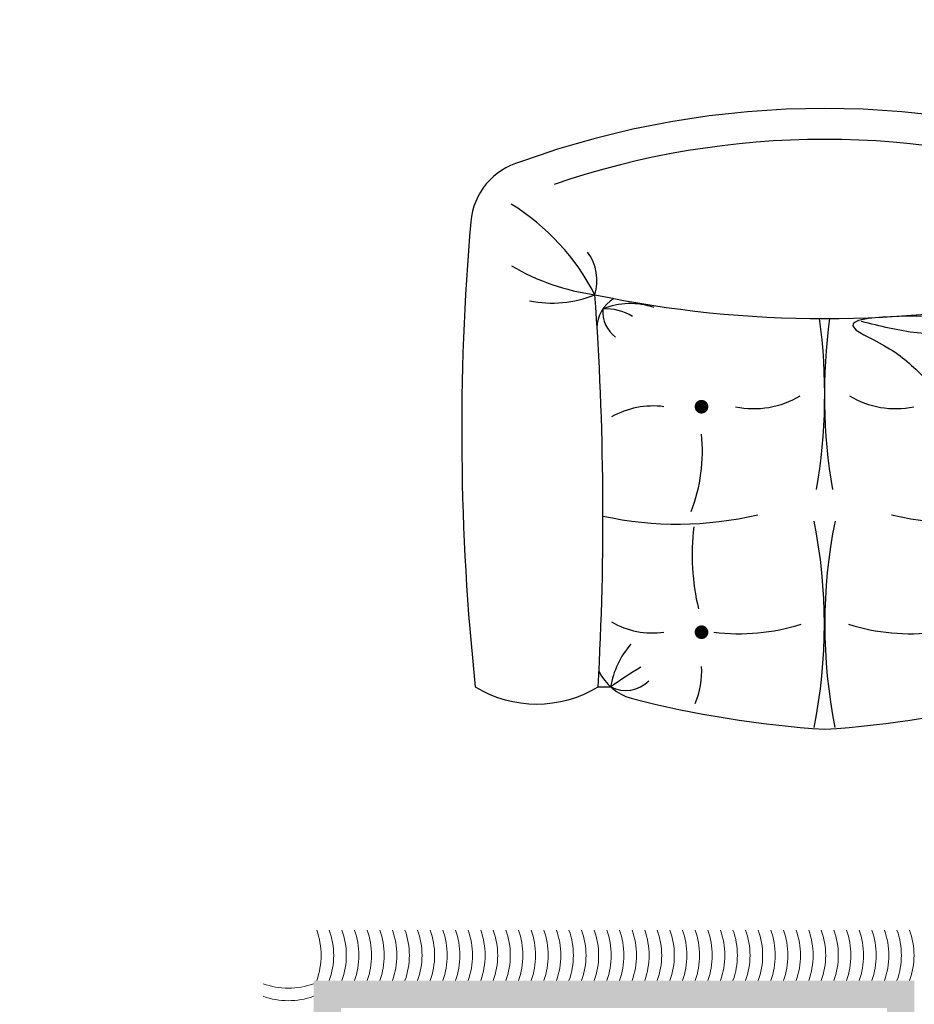
# Model space of a CAD drawing. Units: inches. Extents: x 844 to 2234, y 346 to 1084.
# Tile 88 of 93: x 1990 to 2011, y 713 to 736. Entities that reach past the tile are written whole.
import ezdxf

# ---------------------------------------------------------------- set-up
doc = ezdxf.new("R2010")
doc.units = ezdxf.units.IN
doc.header["$MEASUREMENT"] = 0
for name, color, linetype, lineweight in [('A-ANNO-DIMS', 2, 'Continuous', 18), ('furniture', 8, 'Continuous', 18), ('RA-AP-01$0$INT', 35, 'Continuous', 5)]:
    doc.layers.add(name, color=color, linetype=linetype, lineweight=lineweight)
doc.layers.add('RA-AP-01$0$FURN', color=3, linetype='Continuous')
doc.layers.add('RA-AP-01$0$WOOD', color=64, linetype='Continuous')
doc.styles.get("Standard").update_dxf_attribs({"font": 'arial.ttf'})
doc.dimstyles.get("Standard").update_dxf_attribs({"dimtxt": 6, "dimasz": 3, "dimexe": 0.18, "dimexo": 0.0625, "dimgap": 0.09, "dimtad": 0, "dimtih": 1, "dimtoh": 1, "dimdec": 1, "dimzin": 0, "dimdsep": 46, "dimlunit": 3, "dimtxsty": 'Standard', "dimblk": 'ARCHTICK', "dimcen": 0.09, "dimadec": 0, "dimazin": 0, "dimtfac": 1, "dimtdec": 1, "dimtofl": 0, "dimtmove": 0, "dimatfit": 3, "dimfxl": 1, "dimtolj": 1, "dimtzin": 0, "dimarcsym": 0})

# ---------------------------------------------------------------- blocks, each defined once
blk = doc.blocks.new('A$C18D01794')
at = {"layer": 'RA-AP-01$0$INT'}
h = blk.add_hatch(color=256, dxfattribs=at)
h.paths.add_polyline_path([(4.355206456958071, -6.156712009588037), (4.355206456958071, -8.056712009588038), (5.455206456958072, -8.056712009588038), (5.455206456958072, -6.156712009588037)])
h.paths.add_polyline_path([(4.405206456958072, -8.006712009588039), (4.405206456958072, -6.206712009588038), (5.405206456958072, -6.206712009588038), (5.405206456958072, -8.006712009588039)], flags=16)
for centre, start, end in [((5.501406456971106, -8.156264458284674), 70.20384312943132, 109.796156871843), ((4.492158905671144, -8.102912009578965), 160.2038431286875, 199.7961568711004), ((4.515258905666937, -8.102912009582035), 160.2038431286875, 199.7961568711004), ((4.53835890566273, -8.102912009585104), 160.2038431286875, 199.7961568711004), ((4.561458905665799, -8.102912009585218), 160.2038431286875, 199.7961568711004), ((4.584558905661592, -8.102912009588287), 160.2038431286875, 199.7961568711004), ((4.607658905664661, -8.102912009588401), 160.2038431286875, 199.7961568711004), ((4.630758905664774, -8.102912009585673), 160.2038431286875, 199.7961568711004), ((4.653858905660567, -8.102912009588742), 160.2038431286875, 199.7961568711004), ((4.676958905663636, -8.102912009588856), 160.2038431286875, 199.7961568711004), ((4.700058905663976, -8.102912009589083), 160.2038431286875, 199.7961568711004), ((4.723158905662498, -8.102912009586241), 160.2038431286875, 199.7961568711004), ((4.746258905662839, -8.102912009586355), 160.2038431286875, 199.7961568711004), ((4.769358905662952, -8.102912009589536), 160.2038431286875, 199.7961568711004), ((4.792458905660109, -8.102912009586696), 160.2038431286875, 199.7961568711004), ((4.815558905661814, -8.10291200958681), 160.2038431286875, 199.7961568711004), ((4.838658905662154, -8.102912009587037), 160.2038431286875, 199.7961568711004), ((4.861758905665223, -8.102912009590106), 160.2038431286875, 199.7961568711004), ((4.884858905661016, -8.102912009587264), 160.2038431286875, 199.7961568711004), ((4.907958905662721, -8.102912009587492), 160.2038431286875, 199.7961568711004), ((4.931058905658514, -8.102912009590447), 160.2038431286875, 199.7961568711004), ((4.954158905661583, -8.102912009587717), 160.2038431286875, 199.7961568711004), ((4.977258905663288, -8.102912009587946), 160.2038431286875, 199.7961568711004), ((5.000358905663628, -8.102912009587946), 160.2038431286875, 199.7961568711004), ((5.023458905665333, -8.10291200959113), 160.2038431286875, 199.7961568711004), ((5.046558905660899, -8.102912009588287), 160.2038431286875, 199.7961568711004), ((5.069658905661239, -8.102912009588401), 160.2038431286875, 199.7961568711004), ((5.092758905664308, -8.102912009588628), 160.2038431286875, 199.7961568711004), ((5.115858905663057, -8.102912009585786), 160.2038431286875, 199.7961568711004), ((5.13895890566317, -8.102912009588856), 160.2038431286875, 199.7961568711004), ((5.162058905663511, -8.102912009589083), 160.2038431286875, 199.7961568711004), ((5.185158905659076, -8.102912009589197), 160.2038431286875, 199.7961568711004), ((5.208258905660781, -8.102912009586355), 160.2038431286875, 199.7961568711004), ((5.231358905662486, -8.102912009589536), 160.2038431286875, 199.7961568711004), ((5.254458905661235, -8.102912009589652), 160.2038431286875, 199.7961568711004), ((5.277558905661575, -8.102912009589765), 160.2038431286875, 199.7961568711004), ((5.300658905661689, -8.102912009587037), 160.2038431286875, 199.7961568711004), ((5.323758905658846, -8.10291200958715), 160.2038431286875, 199.7961568711004), ((5.346858905659186, -8.10291200959022), 160.2038431286875, 199.7961568711004), ((5.369958905662255, -8.102912009587492), 160.2038431286875, 199.7961568711004), ((5.39305890566396, -8.102912009587492), 160.2038431286875, 199.7961568711004), ((5.416158905664301, -8.102912009587717), 160.2038431286875, 199.7961568711004), ((5.439258905666005, -8.102912009590902), 160.2038431286875, 199.7961568711004), ((5.462358905661571, -8.102912009587946), 160.2038431286875, 199.7961568711004), ((5.485458905657364, -8.10291200958499), 160.2038431286875, 199.7961568711004), ((5.508558905660433, -8.102912009588287), 160.2038431286875, 199.7961568711004), ((5.531658905655999, -8.102912009585332), 160.2038431286875, 199.7961568711004), ((5.554758905651792, -8.102912009582376), 160.2038431286875, 199.7961568711004), ((5.577858905654861, -8.102912009585673), 160.2038431286875, 199.7961568711004), ((5.501406456971106, -8.179364458283423), 70.20384312943132, 109.796156871843)]:
    blk.add_arc(centre, 0.136414042854523, start, end, dxfattribs=at)
blk = doc.blocks.new('A$C7F4351E2')
at = {"layer": 'RA-AP-01$0$FURN'}
for p, q in [((8.352559572600457, -8.263941955512525), (8.35255957259913, -8.282283310927069)), ((8.352559572600457, -8.927748273106442), (8.35255957259913, -8.909406917691898))]:
    blk.add_line(p, q, dxfattribs=at)
at = {"layer": 'RA-AP-01$0$FURN', "const_width": 0.01}
for points in [[(8.437812509519787, -8.415359762755768, 1), (8.427812509519786, -8.415359762755742, 1)], [(8.758197489244363, -8.415359762756214, -1), (8.768197489244365, -8.415359762756214, -1)], [(8.437812509519787, -8.776330465863198, -1), (8.427812509519786, -8.776330465863225, -1)], [(8.758197489244363, -8.776330465862753, 1), (8.768197489244365, -8.776330465862753, 1)]]:
    blk.add_lwpolyline(points, format="xyb", close=True, dxfattribs=at)
at = {"layer": 'RA-AP-01$0$FURN'}
for centre, radius, start, end in [((8.727559572604601, -11.61690445537682), 3.552808610866049, 85.0473312316413, 96.05887237565803), ((9.025650106946005, -8.176987401637472), 0.1, 15.499494600857, 85.04733123164159), ((8.50205957259015, -8.17394195551301), 0.1744999999876311, 148.9517780040467, 211.048221995953), ((8.77247054904813, -7.958543863781743), 0.3382138395168437, 297.2303327094027, 328.2563708342649), ((9.2484631175852, -8.302692737637487), 0.3241573581843151, 149.2985674842688, 172.3026350986055), ((7.88981694267423, -8.595845114309485), 1.310286319972027, 340.1192502251003, 19.8807497748998), ((9.084915705374858, -8.196040134964925), 0.1698955038956699, 168.877843135945, 201.8512383801196), ((7.929864357850293, -8.595845114309483), 1.224941341589781, 341.1257460634955, 18.87425393650447), ((8.947672844970796, -8.191835192646359), 0.0704710051510922, 253.1338634205325, 306.4126496157095), ((8.408522229993444, -8.33300072568355), 0.0753785023123622, 115.8745619060558, 163.9833547230034), ((8.603635103111959, -3.79706073025477), 4.473931917517753, 266.7828902523826, 274.1477233631118), ((8.878389979098333, -8.312202545234353), 0.05, 30.14777190425723, 89.99999999905349), ((10.52713941284929, -8.595845114309466), 1.634931324962266, 168.1200364254424, 191.8799635745573), ((9.101231010340802, -8.38034106221356), 0.5100538472773755, 167.6182489359307, 193.3122231353938), ((8.903279781571525, -8.31837865610295), 0.0478550828899777, 86.575295631534, 142.6833829238214), ((8.838100984994732, -8.276822957859652), 0.0683206773889159, 326.6729861493449, 5.218395042636973), ((8.810121490949696, -8.31110757721543), 0.1042084262671507, 340.4828318717155, 22.86929393278168), ((8.395364730619693, -8.304213854581548), 0.0479292786975047, 152.8070868543555, 225.4025460716553), ((8.333592787569726, -8.402663469525104), 0.1218651776285568, 48.0375529564433, 81.04623209541253), ((7.439612310514541, -8.913795367824825), 1.11020813118073, 31.93286085977143, 34.66647731879807), ((8.553131949433, -8.344109762755968), 0.1214118203512435, 150.1419074485596, 187.691663289156), ((8.642878049331348, -8.344109762756093), 0.1214118203512435, 352.3083367106845, 29.85809255128089), ((9.82633505008426, -8.696671375220811), 1.539060359583382, 165.5338783218257, 176.2437734318419), ((8.374918524725835, -8.294321202996931), 0.1212957045587361, 247.3375839744822, 273.7314750942433), ((8.546954810732721, -8.753394424755975), 0.3517162425384579, 83.41248966761125, 103.1674570565571), ((8.697701155637269, -8.172468128267624), 0.2442261434243043, 248.9017070735605, 275.9923925191661), ((8.73287643248165, -8.469775898206471), 0.3023568492824586, 173.0944825511667, 197.588060785551), ((8.889871101981017, -8.492307869305423), 0.1295083186917369, 167.9901339202812, 211.3796151021958), ((8.444145567704187, -7.829943385268752), 0.765467899454341, 258.6273206109321, 281.4174148186357), ((9.82633505008426, -8.495018853398156), 1.539060359583382, 183.7562265681581, 194.4661216781742), ((8.444145567704187, -9.361312955433425), 0.765467899454341, 78.58258518136427, 101.3726793890678), ((8.781211457338294, -7.772561243483908), 0.8232838708255751, 260.2449188973366, 277.7495311655964), ((8.781211457338294, -9.418695097218269), 0.8232838708255751, 82.25060502413102, 99.75508110266344), ((8.73287643248165, -8.721914330412496), 0.3023568492824586, 162.411939214449, 186.9055174488332), ((8.889871101981017, -8.699382359313544), 0.1295083186917369, 148.6203848978042, 192.0098660797188), ((9.101231010340802, -8.811349166405407), 0.5100538472773755, 166.6877768646062, 192.3817510640693), ((8.799643412436344, -8.749969313933361), 0.0689028341546707, 265.5384273543114, 353.5804828909086), ((8.374918524725835, -8.897369025622035), 0.1212957045587361, 86.26852490575668, 112.6624160255178), ((8.546954810732721, -8.438295803862992), 0.3517162425384579, 256.8325429434429, 276.5875103323888), ((8.697701155637269, -9.019222100351342), 0.2442261434243043, 84.00760748083387, 111.0982929264395), ((8.553131949433, -8.847580465862999), 0.1214118203512435, 172.308336710844, 209.8580925514404), ((8.395364730619693, -8.88747637403742), 0.0479292786975047, 134.5974539283447, 207.1929131456445), ((8.785133372574222, -8.874256642962408), 0.0310151388417235, 42.62105484496073, 114.2239681486109), ((8.810121490949696, -8.880582651403534), 0.1042084262671507, 337.1307060672183, 19.51716812828453), ((7.439612310514541, -8.277894860794142), 1.11020813118073, 325.333522681202, 328.0671391402286), ((8.408522229993444, -8.858689502935416), 0.0753785023123622, 196.0166452769965, 244.1254380939442), ((8.333592787569726, -8.789026759093863), 0.1218651776285568, 278.9537679045875, 311.9624470435567), ((8.838100984994732, -8.914867270759315), 0.0683206773889159, 354.781604957363, 33.32701385065517), ((8.642878049331348, -8.847580465862874), 0.1214118203512435, 330.1419074487191, 340.3913536181062), ((8.878389979098333, -8.879487683384612), 0.05, 270.0000000009465, 337.4173275753961), ((8.903279781571525, -8.873311572516016), 0.0478550828899777, 217.3166170761785, 273.424704368466), ((8.50205957259015, -9.017748273105955), 0.1744999999876311, 148.9517780040469, 211.0482219959533), ((8.603635103111959, -13.39462949836419), 4.473931917517753, 85.85227663688822, 93.21710974761734), ((9.084915705374858, -8.995650093654042), 0.1698955038956699, 158.1487616198804, 191.122156864055), ((8.947672844970796, -8.999855035972608), 0.0704710051510922, 53.58735038429053, 106.8661365794674), ((8.77247054904813, -9.233146364837223), 0.3382138395168437, 31.74362916573515, 62.76966729059727), ((9.2484631175852, -8.88899749098148), 0.3241573581843151, 187.6973649013944, 210.7014325157311), ((9.025650106946005, -9.014702826981493), 0.1, 274.9526687683584, 344.500505399143), ((8.727559572604601, -5.574785773242145), 3.552808610866049, 263.941127624342, 274.9526687683587)]:
    blk.add_arc(centre, radius, start, end, dxfattribs=at)
for points, knots in [([(8.764421239581775, -8.929562504990262), (8.755250524728652, -8.881106864374377), (8.74196437992213, -8.810906376383404), (8.80604948961138, -8.740469753734786), (8.847474678848357, -8.701097198289744), (8.897142214037096, -8.58322730303861), (8.897091569728207, -8.784804210134517), (8.88612504526093, -8.897825917224484), (8.806539053396843, -8.9185794820093), (8.764421239581775, -8.92956250499026)], [0, 0, 0, 0, 0.1367586589314792, 0.1981301758052368, 0.2677729570689282, 0.3281194902553322, 0.4737578340741565, 0.5765194025309516, 0.6920332287422236, 0.6920332287422236, 0.6920332287422236, 0.6920332287422236]), ([(8.764421239581775, -8.92956250499026), (8.782204778269502, -8.914603263160053), (8.821592007255505, -8.881471326160916), (8.86917941606436, -8.814322636989944), (8.867818990542759, -8.729338202119969), (8.881231406199264, -8.676770566934765), (8.888101821971249, -8.649843164808122)], [0, 0, 0, 0, 0.070018540671015, 0.1550780383534498, 0.2344491945777043, 0.3178048737568289, 0.3178048737568289, 0.3178048737568289, 0.3178048737568289])]:
    blk.add_open_spline(points, degree=3, knots=knots, dxfattribs=at)
blk = doc.blocks.new('A$C5D2F253E')
at = {"layer": 'RA-AP-01$0$FURN', "xscale": -0.7999999999883585, "yscale": 0.7999999999883585, "zscale": 0.8, "rotation": 90}
blk.add_blockref('A$C18D01794', (-5.687757199772477, 4.75791982714071), dxfattribs=at)
at = {"layer": 'RA-AP-01$0$WOOD', "xscale": -1, "rotation": 180}
blk.add_blockref('A$C7F4351E2', (-7.164808785335935, -7.45332973198748), dxfattribs=at)
blk = doc.blocks.new('_ArchTick')
at = {"color": 0, "linetype": 'ByBlock', "const_width": 0.15}
blk.add_lwpolyline([(-0.5, -0.5), (0.5, 0.5)], dxfattribs=at)
blk = doc.blocks.new('*D121')
at = {"layer": 'A-ANNO-DIMS', "color": 0, "lineweight": -2, "transparency": 16777216}
for p, q in [((2030.271987351997, 734.262611118704), (2040.245275089302, 734.262611118704)), ((2040.065275089302, 734.262611118704), (2040.065275089302, 704.6043509484256)), ((2040.065275089302, 668.557359536674), (2040.065275089302, 698.2156197069523)), ((2030.271987351997, 668.557359536674), (2040.245275089302, 668.557359536674))]:
    blk.add_line(p, q, dxfattribs=at)
at = {"layer": 'Defpoints', "color": 0, "transparency": 16777216}
for p in [(2030.209487351997, 734.262611118704), (2040.065275089302, 734.262611118704), (2030.209487351997, 668.557359536674)]:
    blk.add_point(p, dxfattribs=at)
at = {"layer": 'A-ANNO-DIMS', "color": 0, "lineweight": -2, "transparency": 16777216, "xscale": 3, "yscale": 3, "zscale": 3}
for p, rotation in [((2040.065275089302, 734.262611118704), 90), ((2040.065275089302, 668.557359536674), 270)]:
    blk.add_blockref('_ArchTick', p, dxfattribs=dict(at, rotation=rotation))
at = {"layer": 'A-ANNO-DIMS', "color": 0, "transparency": 16777216, "insert": (2040.065275089302, 701.4099853276883), "char_height": 6, "attachment_point": 5}
blk.add_mtext('\\A1;LOUNGE SET 5\'-5 1/2" TYP.', dxfattribs=at)

msp = doc.modelspace()

# ---------------------------------------------------------------- block references
at = {"layer": 'furniture', "xscale": -15.94108302203742, "yscale": 15.94108302203742, "zscale": 15.94108302203742, "rotation": 270}
msp.add_blockref('A$C5D2F253E', (1990.567271852805, 701.4028671565849), dxfattribs=at)

# ---------------------------------------------------------------- dimensions: what is measured, and where the dimension line sits
at = {"layer": 'A-ANNO-DIMS'}
dim = msp.add_linear_dim(base=(2040.065275089302, 734.262611118704), p1=(2030.209487351996, 668.5573595366737), p2=(2030.209487351996, 734.2626111187037), angle=90, text='LOUNGE SET <> TYP.', dimstyle='Standard', override={"dimdec": 1, "dimlfac": 1, "dimrnd": 0, "dimzin": 1, "dimdsep": 46, "dimlunit": 4, "dimfrac": 2}, dxfattribs=at)
dim.commit()
dim.dimension.update_dxf_attribs({"geometry": '*D121', "text_midpoint": (2040.065275089302, 701.4099853276883)})

doc.saveas('drawing.dxf')
